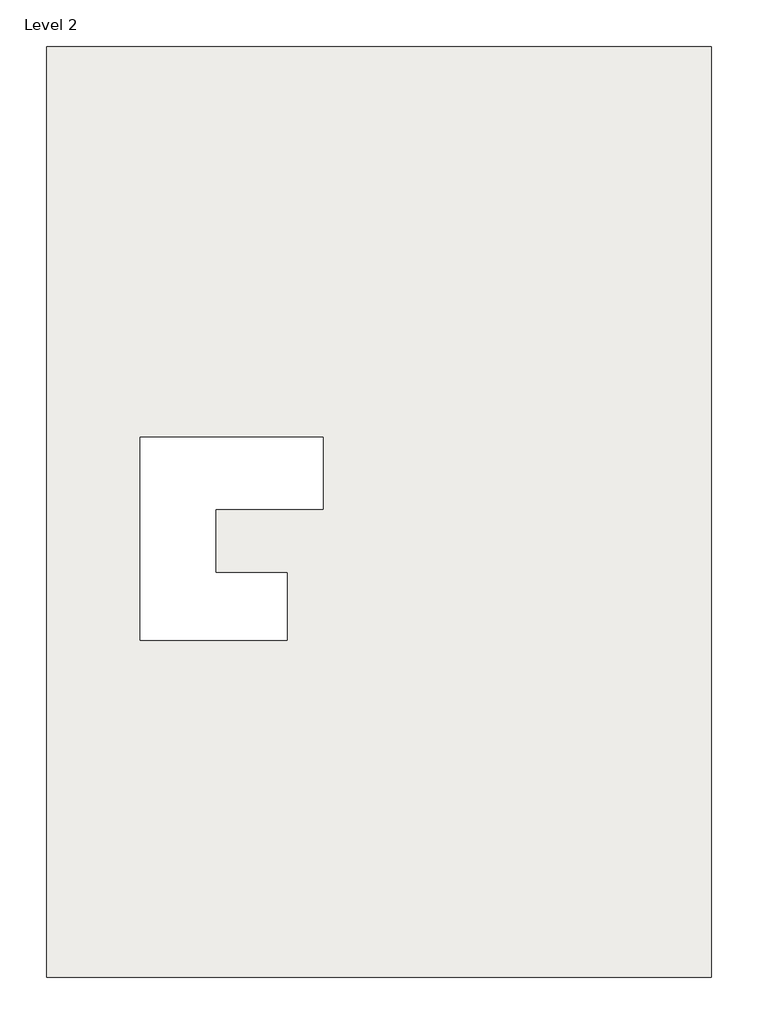
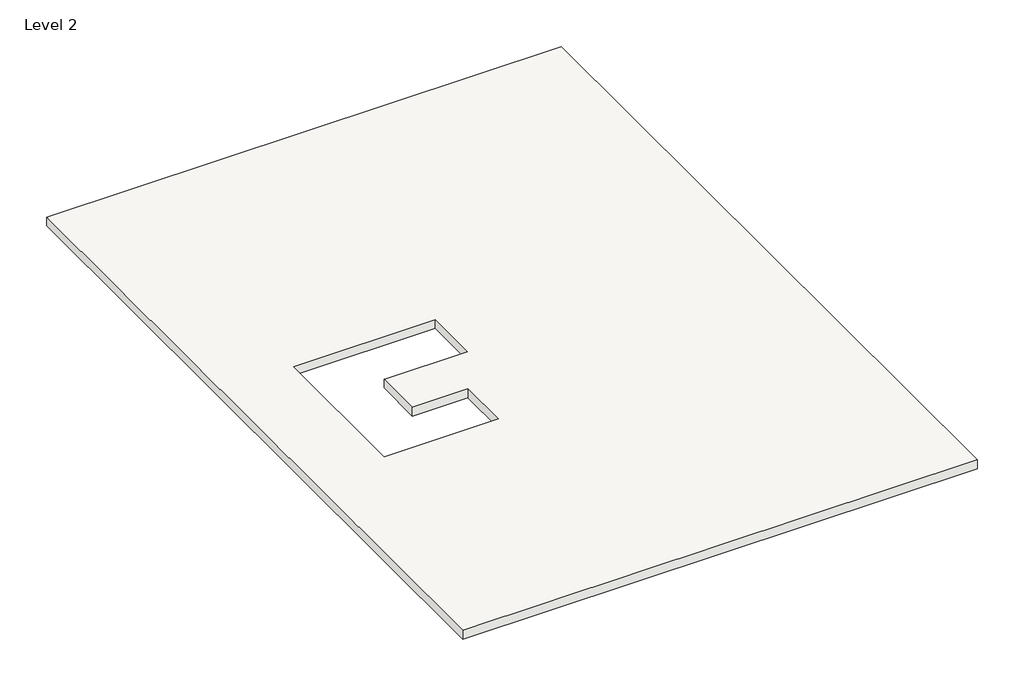
# One storey, incomplete: 1 roof.
"""IFC4 building model written with IfcOpenShell, lengths in millimetres."""

from ifc_helpers import new_model, si_unit, frame, origin, place, context, project, spatial, polyline, outline, extrude, element, save

model = new_model("IFC4")

# Units and contexts
model_context = context("Model", 3, world=origin())
ifc_project = project(units=[si_unit("LENGTHUNIT", "METRE", prefix="MILLI")], contexts=[model_context])

# Site, building, storey
site = spatial("IfcSite", under=ifc_project)
building = spatial("IfcBuilding", under=site)
storey = spatial("IfcBuildingStorey", under=building, Name="Level 2", Elevation=3048.0)

# Roof
placement = place(None, origin())
element("IfcRoof", 1, ObjectType="ROOF 6\"", at=placement, inside=storey, context=model_context, shape_type="SweptSolid", body=[
    extrude(outline(polyline([(-7082.9340247, 5913.1319954), (1413.3659753, 5913.1319954), (1413.3659753, -5974.0680046), (-7082.9340247, -5974.0680046), (-7082.9340247, 5913.1319954)]), holes=[polyline([(-5889.1340247, 922.0319954), (-5889.1340247, -1668.7680046), (-4009.5340247, -1668.7680046), (-4009.5340247, -805.1680046), (-4923.9340247, -805.1680046), (-4923.9340247, 7.6319954), (-3552.3340247, 7.6319954), (-3552.3340247, 922.0319954), (-5889.1340247, 922.0319954)])]), frame((0.0, 0.0, 3048.0), z_axis=(0.0, 0.0, 1.0), x_axis=(1.0, 0.0, 0.0)), (0.0, 0.0, 1.0), 152.4),
])

save(model, "model.ifc")

# Revit data of these elements
# Type "ROOF 6\""
#   Assembly Code = "B1020"
#   Layers, outside or top first: 0' - 6" no material (function 1)
# Element 1 (IfcRoof, "ROOF 6\"")
#   built-in parameter 1001705 = 10.5 (stored number, unit not read)
#   built-in parameter 1001710 = 33615
#   Phase Created = New Construction
#   Materials on its faces: "Default Roof", "Oak Flooring"
# Materials
#   "Default Roof": colour RGB 88 101 114, transparency 0, Cost = 0
#   "Oak Flooring": class "Wood", colour RGB 216 169 114, transparency 0, Description = "Quercus Rubra", Cost = 0
